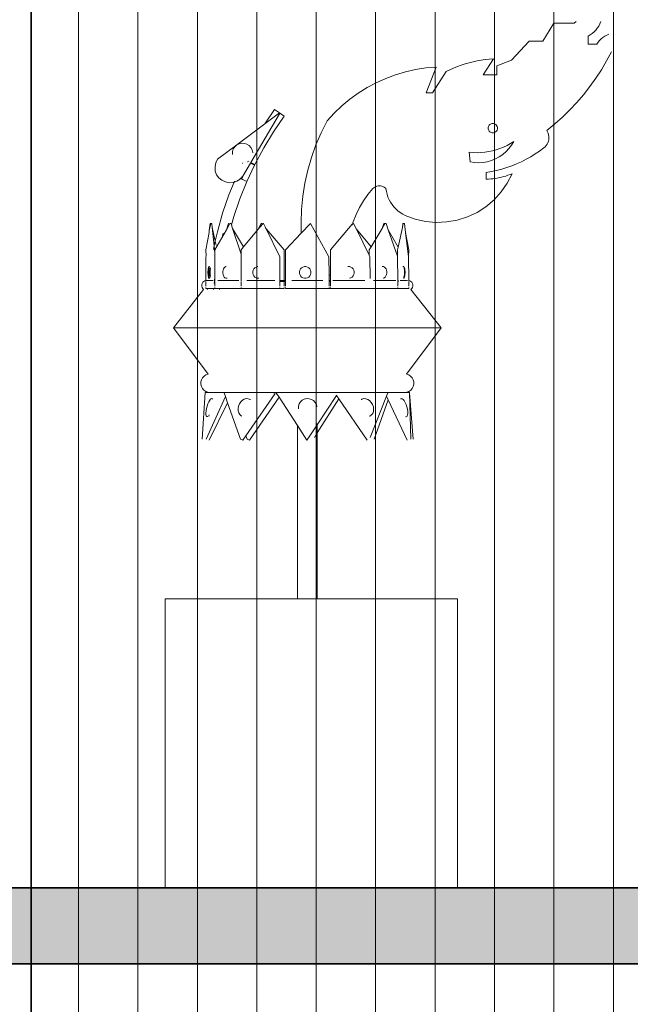
# Model space of a CAD drawing. Units: millimetres. Extents: x 446512 to 447461, y 70395 to 70610.
# Tile 24 of 39: x 446983 to 447016, y 70477 to 70530. Entities that reach past the tile are written whole.
import ezdxf

# ---------------------------------------------------------------- set-up
doc = ezdxf.new("R2010")
doc.units = ezdxf.units.MM
for name, color, linetype, lineweight in [('A-FURN', 7, 'Continuous', 35), ('A-FURN-DECO', 8, 'Continuous', 13), ('A-FURN-PATT', 38, 'Continuous', 13)]:
    doc.layers.add(name, color=color, linetype=linetype, lineweight=lineweight)

msp = doc.modelspace()

# ---------------------------------------------------------------- hatches: boundary and pattern name
at = {"layer": 'A-FURN-PATT'}
h = msp.add_hatch(dxfattribs=at)
h.set_pattern_fill('ANSI31', color=256, angle=45)
h.paths.add_polyline_path([(447044.0961, 70599.7147), (446983.5069, 70599.7147), (446983.5069, 70556.4508), (447030.1693, 70556.4508), (447030.1693, 70442.4508), (446983.5069, 70442.4508), (446983.5069, 70405.3145), (447044.0961, 70405.3145)])
h.paths.add_polyline_path([(447021.1693, 70547.4508), (446983.5069, 70547.4508), (446983.5069, 70451.4508), (447021.1693, 70451.4508)], flags=17)
h = msp.add_hatch(color=256, dxfattribs=at)
h.dxf.hatch_style = 1
h.paths.add_polyline_path([(447021.1693, 70483.6935), (446983.5069, 70483.6935), (446983.5069, 70479.6272), (447021.1693, 70479.6272)], flags=17)
h.paths.add_polyline_path([(447030.1693, 70483.6935), (447021.1693, 70483.6935), (447021.1693, 70479.6272), (447030.1693, 70479.6272)], flags=17)
h.paths.add_polyline_path([(447044.0961, 70599.7147), (446983.5069, 70599.7147), (446983.5069, 70556.4508), (447030.1693, 70556.4508), (447030.1693, 70442.4508), (446983.5069, 70442.4508), (446983.5069, 70405.3145), (447044.0961, 70405.3145)])
h = msp.add_hatch(color=256, dxfattribs=at)
h.dxf.hatch_style = 1
h.paths.add_polyline_path([(446983.5069, 70483.6935), (446973.1693, 70483.6935), (446973.1693, 70479.6272), (446983.5069, 70479.6272)])

# ---------------------------------------------------------------- linework, layer by layer
at = {"layer": 'A-FURN'}
for p, q in [((446983.5069, 70599.7147), (446983.5069, 70405.3145)), ((446990.6642, 70483.6935), (447006.2723, 70483.6935))]:
    msp.add_line(p, q, dxfattribs=at)
msp.add_lwpolyline([(446964.1693, 70483.6935), (447030.1693, 70483.6935), (447030.1693, 70479.6272), (446964.1693, 70479.6272)], close=True, dxfattribs=at)
at = {"layer": 'A-FURN-DECO'}
for p, q in [((447010.828, 70528.8929), (447011.4196, 70529.8484)), ((447011.4196, 70529.8484), (447012.5122, 70529.8484)), ((447012.5122, 70529.8484), (447012.6141, 70529.9403)), ((447013.7432, 70529.5803), (447013.6614, 70529.477)), ((447013.815, 70529.6908), (447013.7432, 70529.5803)), ((447013.8759, 70529.8076), (447013.815, 70529.6908)), ((447013.9256, 70529.9297), (447013.8759, 70529.8076)), ((447013.3629, 70529.2196), (447013.2487, 70529.1538)), ((447013.2487, 70529.1538), (447013.2487, 70528.7324)), ((447013.4704, 70529.2958), (447013.3629, 70529.2196)), ((447013.5702, 70529.3819), (447013.4704, 70529.2958)), ((447013.6614, 70529.477), (447013.5702, 70529.3819)), ((447013.8599, 70528.9241), (447013.9447, 70529.0087)), ((447013.9447, 70529.0087), (447014.0372, 70529.0847)), ((447014.0372, 70529.0847), (447014.1366, 70529.1514)), ((447014.1366, 70529.1514), (447014.242, 70529.2082)), ((447014.242, 70529.2082), (447014.3524, 70529.2545)), ((447009.1665, 70527.8803), (447010.0944, 70528.8929)), ((447010.0944, 70528.8929), (447010.828, 70528.8929)), ((447013.2487, 70528.7324), (447013.7169, 70528.7324)), ((447013.7169, 70528.7324), (447013.7838, 70528.8317)), ((447013.7838, 70528.8317), (447013.8599, 70528.9241)), ((447008.1897, 70527.9357), (447007.6509, 70527.0946)), ((447007.7535, 70527.9005), (447007.9713, 70527.922)), ((447007.9713, 70527.922), (447008.1897, 70527.9357)), ((447014.4944, 70528.3187), (447014.2376, 70527.8352)), ((447004.0349, 70527.3713), (447004.5847, 70527.4558)), ((447004.5847, 70527.4558), (447005.139, 70527.5027)), ((447005.139, 70527.5027), (447004.5947, 70526.1235)), ((447005.867, 70527.3633), (447006.0668, 70527.4527)), ((447006.0668, 70527.4527), (447006.2696, 70527.5349)), ((447006.2696, 70527.5349), (447006.4753, 70527.6097)), ((447006.4753, 70527.6097), (447006.6835, 70527.6771)), ((447006.6835, 70527.6771), (447006.8941, 70527.7371)), ((447006.8941, 70527.7371), (447007.1066, 70527.7894)), ((447007.1066, 70527.7894), (447007.3208, 70527.8342)), ((447007.3208, 70527.8342), (447007.5366, 70527.8712)), ((447007.5366, 70527.8712), (447007.7535, 70527.9005)), ((447008.3689, 70527.5628), (447009.1665, 70527.8803)), ((447008.3689, 70527.0946), (447008.3689, 70527.5628)), ((447014.2376, 70527.8352), (447013.9594, 70527.3635)), ((447001.9306, 70526.6685), (447002.4375, 70526.8975)), ((447002.4375, 70526.8975), (447002.9588, 70527.0915)), ((447002.9588, 70527.0915), (447003.4921, 70527.2497)), ((447003.4921, 70527.2497), (447004.0349, 70527.3713)), ((447004.9381, 70526.1235), (447005.6705, 70527.2669)), ((447005.6705, 70527.2669), (447005.867, 70527.3633)), ((447007.6509, 70527.0946), (447008.3689, 70527.0946)), ((447013.6605, 70526.9048), (447013.3415, 70526.4598)), ((447013.9594, 70527.3635), (447013.6605, 70526.9048)), ((447000.9691, 70526.1101), (447001.4403, 70526.4057)), ((447001.4403, 70526.4057), (447001.9306, 70526.6685)), ((447013.3415, 70526.4598), (447013.0029, 70526.0295)), ((447000.519, 70525.7833), (447000.9691, 70526.1101)), ((447004.5947, 70526.1235), (447004.9381, 70526.1235)), ((447013.0029, 70526.0295), (447012.6455, 70525.6147)), ((446999.6905, 70525.0418), (447000.0921, 70525.4266)), ((447000.0921, 70525.4266), (447000.519, 70525.7833)), ((447012.6455, 70525.6147), (447012.2699, 70525.2162)), ((446996.7604, 70525.015), (446995.2353, 70522.4145)), ((446996.5029, 70525.2318), (446995.9841, 70524.4744)), ((446996.7604, 70525.0554), (446995.9841, 70524.4744)), ((446996.4467, 70524.0451), (446997.018, 70524.879)), ((446996.7604, 70525.0554), (446996.5029, 70525.2318)), ((446996.7604, 70525.015), (446996.7604, 70525.0554)), ((446997.018, 70524.879), (446996.7604, 70525.0554)), ((446999.3159, 70524.6306), (446999.6905, 70525.0418)), ((447011.8769, 70524.8349), (447011.4674, 70524.4715)), ((447012.2699, 70525.2162), (447011.8769, 70524.8349)), ((446995.9841, 70524.4744), (446994.4826, 70523.344)), ((446999.3159, 70524.6306), (446998.9957, 70523.9976)), ((447007.9127, 70524.2101), (447007.913, 70524.2753)), ((447007.913, 70524.2753), (447007.9302, 70524.3381)), ((447007.9302, 70524.3381), (447007.9631, 70524.3944)), ((447007.9631, 70524.3944), (447008.0095, 70524.4403)), ((447008.0095, 70524.4403), (447008.0661, 70524.4726)), ((447008.0661, 70524.4726), (447008.1291, 70524.4891)), ((447008.1291, 70524.4891), (447008.1943, 70524.4888)), ((447008.1943, 70524.4888), (447008.2572, 70524.4716)), ((447008.2572, 70524.4716), (447008.3135, 70524.4387)), ((447008.3135, 70524.4387), (447008.3594, 70524.3924)), ((447008.3594, 70524.3924), (447008.3917, 70524.3358)), ((447008.3917, 70524.3358), (447008.4082, 70524.2727)), ((447008.4082, 70524.2727), (447008.4079, 70524.2075)), ((447011.4674, 70524.4715), (447011.042, 70524.1267)), ((446995.9258, 70523.1888), (446996.4467, 70524.0451)), ((446998.9957, 70523.9976), (446998.7153, 70523.3461)), ((447007.9292, 70524.147), (447007.9127, 70524.2101)), ((447007.9616, 70524.0904), (447007.9292, 70524.147)), ((447008.0074, 70524.044), (447007.9616, 70524.0904)), ((447008.0637, 70524.0112), (447008.0074, 70524.044)), ((447008.1266, 70523.994), (447008.0637, 70524.0112)), ((447008.1918, 70523.9936), (447008.1266, 70523.994)), ((447008.2548, 70524.0102), (447008.1918, 70523.9936)), ((447008.3115, 70524.0425), (447008.2548, 70524.0102)), ((447008.3578, 70524.0883), (447008.3115, 70524.0425)), ((447008.3907, 70524.1446), (447008.3578, 70524.0883)), ((447008.4079, 70524.2075), (447008.3907, 70524.1446)), ((447011.042, 70524.1267), (447011.0855, 70524.0511)), ((447011.0855, 70524.0511), (447011.1192, 70523.9707)), ((447011.1192, 70523.9707), (447011.1426, 70523.8866)), ((447011.1426, 70523.8866), (447011.1554, 70523.8004)), ((447011.1573, 70523.7131), (447011.1484, 70523.6264)), ((447011.1554, 70523.8004), (447011.1573, 70523.7131)), ((446994.4826, 70523.344), (446993.4537, 70522.5809)), ((446994.2989, 70523.1363), (446994.3766, 70523.2518)), ((446994.3766, 70523.2518), (446994.4826, 70523.344)), ((446994.4826, 70523.344), (446994.6097, 70523.4065)), ((446994.6097, 70523.4065), (446994.7492, 70523.4351)), ((446994.7492, 70523.4351), (446994.8916, 70523.4278)), ((446994.8916, 70523.4278), (446995.0273, 70523.3852)), ((446995.0273, 70523.3852), (446995.1468, 70523.3101)), ((446995.1468, 70523.3101), (446995.2422, 70523.2077)), ((446995.2422, 70523.2077), (446995.3069, 70523.085)), ((446995.9258, 70523.1888), (446995.4519, 70522.3056)), ((446998.7153, 70523.3461), (446998.4757, 70522.6785)), ((447008.7364, 70523.2332), (447008.5432, 70523.1548)), ((447008.9247, 70523.3227), (447008.7364, 70523.2332)), ((447009.1074, 70523.4232), (447008.9247, 70523.3227)), ((447009.1636, 70523.3387), (447009.0236, 70523.1569)), ((447009.2838, 70523.5343), (447009.1074, 70523.4232)), ((447009.2838, 70523.5343), (447009.1636, 70523.3387)), ((447010.8853, 70523.1876), (447010.6588, 70523.0208)), ((447010.951, 70523.245), (447010.8853, 70523.1876)), ((447011.009, 70523.3102), (447010.951, 70523.245)), ((447011.0584, 70523.3821), (447011.009, 70523.3102)), ((447011.0985, 70523.4595), (447011.0584, 70523.3821)), ((447011.1287, 70523.5414), (447011.0985, 70523.4595)), ((447011.1484, 70523.6264), (447011.1287, 70523.5414)), ((446994.2473, 70522.8678), (446994.2548, 70523.0053)), ((446994.2484, 70522.8629), (446994.2473, 70522.8678)), ((446994.2473, 70522.8435), (446994.2484, 70522.8629)), ((446994.2548, 70523.0053), (446994.2989, 70523.1363)), ((446995.3069, 70523.085), (446995.3365, 70522.9502)), ((446995.3355, 70522.9308), (446995.3365, 70522.9502)), ((446995.3355, 70522.9308), (446995.3365, 70522.926)), ((446998.4757, 70522.6785), (446998.2778, 70521.9974)), ((447007.1102, 70522.9384), (447006.9025, 70522.9561)), ((447006.9025, 70522.9561), (447006.9537, 70522.4376)), ((447007.3186, 70522.9328), (447007.1102, 70522.9384)), ((447007.527, 70522.9395), (447007.3186, 70522.9328)), ((447007.7346, 70522.9585), (447007.527, 70522.9395)), ((447007.9408, 70522.9896), (447007.7346, 70522.9585)), ((447008.1447, 70523.0329), (447007.9408, 70522.9896)), ((447008.3458, 70523.088), (447008.1447, 70523.0329)), ((447008.5004, 70522.7132), (447008.2982, 70522.6046)), ((447008.5432, 70523.1548), (447008.3458, 70523.088)), ((447008.6901, 70522.8424), (447008.5004, 70522.7132)), ((447008.8651, 70522.9908), (447008.6901, 70522.8424)), ((447009.0236, 70523.1569), (447008.8651, 70522.9908)), ((447010.1858, 70522.7165), (447009.9402, 70522.5794)), ((447010.4255, 70522.8637), (447010.1858, 70522.7165)), ((447010.6588, 70523.0208), (447010.4255, 70522.8637)), ((446993.3619, 70522.3972), (446993.3224, 70522.1968)), ((446993.3224, 70522.1564), (446993.3224, 70522.1968)), ((446993.3224, 70522.1564), (446993.338, 70521.953)), ((446993.4537, 70522.5809), (446993.3619, 70522.3972)), ((446994.7995, 70522.3847), (446994.7884, 70522.3611)), ((446995.2135, 70522.3774), (446994.8064, 70521.6831)), ((446995.0294, 70521.4043), (446995.4365, 70522.2728)), ((446995.0554, 70522.4515), (446995.0806, 70522.4397)), ((446995.1245, 70522.4701), (446995.1069, 70522.479)), ((446995.2353, 70522.4145), (446995.2135, 70522.3774)), ((446995.4365, 70522.2728), (446995.2135, 70522.3774)), ((446995.2353, 70522.4145), (446995.4519, 70522.3056)), ((447007.1809, 70522.4055), (447006.9537, 70522.4376)), ((447007.4103, 70522.3976), (447007.1809, 70522.4055)), ((447007.6393, 70522.4139), (447007.4103, 70522.3976)), ((447007.8652, 70522.4541), (447007.6393, 70522.4139)), ((447008.0857, 70522.518), (447007.8652, 70522.4541)), ((447008.2982, 70522.6046), (447008.0857, 70522.518)), ((447008.9067, 70522.1377), (447008.6379, 70522.0548)), ((447009.1718, 70522.2317), (447008.9067, 70522.1377)), ((447009.4327, 70522.3369), (447009.1718, 70522.2317)), ((447009.689, 70522.4528), (447009.4327, 70522.3369)), ((447009.9402, 70522.5794), (447009.689, 70522.4528)), ((446993.338, 70521.953), (446993.4076, 70521.7604)), ((446993.4076, 70521.7604), (446993.5263, 70521.5917)), ((446994.6967, 70521.5603), (446994.8064, 70521.6831)), ((446994.851, 70521.7593), (446994.7467, 70521.5369)), ((446998.2778, 70521.9974), (446998.1223, 70521.3053)), ((447008.0911, 70521.9232), (447007.814, 70521.8748)), ((447007.814, 70521.8748), (447007.814, 70521.5158)), ((447008.3659, 70521.9833), (447008.0911, 70521.9232)), ((447008.6379, 70522.0548), (447008.3659, 70521.9833)), ((447008.514, 70521.6004), (447008.6288, 70521.6265)), ((447008.6288, 70521.6265), (447008.7427, 70521.656)), ((447008.7427, 70521.656), (447008.8557, 70521.6889)), ((447008.8557, 70521.6889), (447008.9677, 70521.725)), ((447009.1882, 70521.8072), (447008.9299, 70521.3024)), ((447008.9677, 70521.725), (447009.0785, 70521.7645)), ((447009.0785, 70521.7645), (447009.1882, 70521.8072)), ((446993.5263, 70521.5917), (446993.6862, 70521.4585)), ((446993.6862, 70521.4585), (446993.8764, 70521.3698)), ((446993.8764, 70521.3698), (446994.0839, 70521.3317)), ((446994.3382, 70521.3615), (446994.0656, 70520.6874)), ((446994.0839, 70521.3317), (446994.2945, 70521.3467)), ((446994.2945, 70521.3467), (446994.3382, 70521.3615)), ((446994.3382, 70521.3615), (446994.4939, 70521.4139)), ((446994.3571, 70521.4083), (446994.3382, 70521.3615)), ((446994.4939, 70521.4139), (446994.6685, 70521.5287)), ((446994.6507, 70520.469), (446995.0265, 70521.3981)), ((446994.655, 70521.5602), (446994.685, 70521.5471)), ((446994.6685, 70521.5287), (446994.685, 70521.5471)), ((446994.6967, 70521.5603), (446994.6736, 70521.5711)), ((446994.685, 70521.5471), (446994.6967, 70521.5603)), ((446994.685, 70521.5471), (446995.0265, 70521.3981)), ((446994.6967, 70521.5603), (446995.0294, 70521.4043)), ((446994.7467, 70521.5369), (446994.7403, 70521.523)), ((446998.1223, 70521.3053), (446998.0099, 70520.605)), ((447001.8507, 70521.0987), (447001.7973, 70521.06)), ((447001.9089, 70521.1296), (447001.8507, 70521.0987)), ((447001.9708, 70521.1521), (447001.9089, 70521.1296)), ((447002.0353, 70521.1657), (447001.9708, 70521.1521)), ((447002.101, 70521.1703), (447002.0353, 70521.1657)), ((447002.1668, 70521.1657), (447002.101, 70521.1703)), ((447002.2313, 70521.1521), (447002.1668, 70521.1657)), ((447002.2932, 70521.1296), (447002.2313, 70521.1521)), ((447002.3514, 70521.0987), (447002.2932, 70521.1296)), ((447002.4048, 70521.06), (447002.3514, 70521.0987)), ((447007.814, 70521.5158), (447007.9315, 70521.5213)), ((447007.9315, 70521.5213), (447008.0489, 70521.5302)), ((447008.0489, 70521.5302), (447008.1659, 70521.5426)), ((447008.1659, 70521.5426), (447008.2825, 70521.5584)), ((447008.2825, 70521.5584), (447008.3986, 70521.5777)), ((447008.3986, 70521.5777), (447008.514, 70521.6004)), ((447008.9299, 70521.3024), (447008.6075, 70520.836)), ((446994.0656, 70520.6874), (446993.7296, 70519.7073)), ((446998.0099, 70520.605), (446997.941, 70519.899)), ((447001.4853, 70520.6969), (447001.2466, 70520.3596)), ((447001.7499, 70521.0143), (447001.4853, 70520.6969)), ((447001.7973, 70521.06), (447001.7499, 70521.0143)), ((447002.4522, 70521.0143), (447002.4048, 70521.06)), ((447002.4749, 70520.8621), (447002.4522, 70521.0143)), ((447002.5107, 70520.7125), (447002.4749, 70520.8621)), ((447002.5595, 70520.5666), (447002.5107, 70520.7125)), ((447002.6207, 70520.4254), (447002.5595, 70520.5666)), ((447008.6075, 70520.836), (447008.2264, 70520.4162)), ((446994.3256, 70519.5208), (446994.6507, 70520.469)), ((447001.2466, 70520.3596), (447001.0353, 70520.0045)), ((447002.694, 70520.2902), (447002.6207, 70520.4254)), ((447002.7787, 70520.1618), (447002.694, 70520.2902)), ((447002.8743, 70520.0413), (447002.7787, 70520.1618)), ((447002.9801, 70519.9295), (447002.8743, 70520.0413)), ((447007.7934, 70520.0502), (447007.3159, 70519.7444)), ((447008.2264, 70520.4162), (447007.7934, 70520.0502)), ((446993.7296, 70519.7073), (446993.447, 70518.7106)), ((446994.1992, 70519.0747), (446994.3256, 70519.5208)), ((446997.941, 70519.899), (446997.9158, 70519.1902)), ((447000.8526, 70519.6339), (447000.6997, 70519.2501)), ((447001.0353, 70520.0045), (447000.8526, 70519.6339)), ((447003.0951, 70519.8274), (447002.9801, 70519.9295)), ((447003.2186, 70519.7357), (447003.0951, 70519.8274)), ((447003.3497, 70519.6551), (447003.2186, 70519.7357)), ((447003.4872, 70519.5862), (447003.3497, 70519.6551)), ((447004.0189, 70519.3891), (447003.4872, 70519.5862)), ((447006.8023, 70519.5041), (447006.2615, 70519.3336)), ((447007.3159, 70519.7444), (447006.8023, 70519.5041)), ((446993.0154, 70518.7719), (446993.0649, 70519.161)), ((446993.0901, 70519.161), (446993.0154, 70518.7719)), ((446993.0901, 70519.161), (446993.0649, 70519.161)), ((446993.0901, 70519.161), (446993.1514, 70519.161)), ((446993.1746, 70518.9378), (446993.1514, 70519.161)), ((446993.93, 70518.8245), (446994.0469, 70519.161)), ((446994.1208, 70519.161), (446993.93, 70518.8245)), ((446994.0614, 70519.161), (446994.0469, 70519.161)), ((446994.1708, 70519.161), (446994.1208, 70519.161)), ((446994.1992, 70519.0747), (446994.1708, 70519.161)), ((446994.2625, 70518.8821), (446994.1992, 70519.0747)), ((446995.6281, 70518.8465), (446995.7833, 70519.161)), ((446995.8507, 70519.1138), (446995.6281, 70518.8465)), ((446995.8106, 70519.161), (446995.7833, 70519.161)), ((446995.8106, 70519.161), (446995.8507, 70519.1138)), ((446995.89, 70519.161), (446995.8507, 70519.1138)), ((446995.9197, 70519.161), (446995.89, 70519.161)), ((446996.0624, 70518.8653), (446995.9197, 70519.161)), ((446997.9158, 70519.1902), (446997.9304, 70518.636)), ((446998.4275, 70519.161), (446997.9304, 70518.636)), ((446999.4032, 70517.382), (446998.4275, 70519.161)), ((447000.6564, 70519.1101), (446999.4869, 70517.7442)), ((447000.6564, 70519.1101), (447000.6445, 70519.0715)), ((447000.6601, 70519.1218), (447000.6564, 70519.1101)), ((447000.6564, 70519.1101), (447000.6668, 70519.0976)), ((447000.6997, 70519.2501), (447000.6601, 70519.1218)), ((447000.6935, 70519.161), (447000.6601, 70519.1218)), ((447000.6935, 70519.161), (447000.7207, 70519.161)), ((447000.8759, 70518.8465), (447000.7207, 70519.161)), ((447002.2416, 70518.8821), (447002.3332, 70519.161)), ((447002.3957, 70519.139), (447002.2416, 70518.8821)), ((447002.3332, 70519.161), (447002.3832, 70519.161)), ((447002.3832, 70519.161), (447002.3957, 70519.139)), ((447002.4088, 70519.161), (447002.3957, 70519.139)), ((447002.4088, 70519.161), (447002.4572, 70519.161)), ((447002.5741, 70518.8245), (447002.4572, 70519.161)), ((447003.3295, 70518.9378), (447003.3526, 70519.161)), ((447003.3784, 70519.161), (447003.3295, 70518.9378)), ((447003.3526, 70519.161), (447003.3784, 70519.161)), ((447003.3784, 70519.161), (447003.4392, 70519.161)), ((447003.4392, 70519.161), (447003.501, 70518.6746)), ((447004.5718, 70519.2638), (447004.0189, 70519.3891)), ((447005.1365, 70519.2124), (447004.5718, 70519.2638)), ((447005.703, 70519.2358), (447005.1365, 70519.2124)), ((447006.2615, 70519.3336), (447005.703, 70519.2358)), ((446993.003, 70518.6746), (446992.8365, 70517.7442)), ((446993.003, 70518.6746), (446993.0154, 70518.7719)), ((446993.1746, 70518.9378), (446993.3341, 70518.2106)), ((446993.2765, 70517.9553), (446993.1746, 70518.9378)), ((446993.93, 70518.8245), (446993.3173, 70517.7442)), ((446993.447, 70518.7106), (446993.3341, 70518.2106)), ((446993.7497, 70518.6335), (446993.702, 70518.4225)), ((446994.2625, 70518.8821), (446994.8465, 70517.908)), ((446994.7101, 70517.5195), (446994.2625, 70518.8821)), ((446995.6281, 70518.8465), (446994.8465, 70517.908)), ((446995.9939, 70518.9457), (446996.0624, 70518.8653)), ((446996.0624, 70518.8653), (446997.0171, 70517.7442)), ((446996.7781, 70517.382), (446996.0624, 70518.8653)), ((446997.9304, 70518.636), (446997.0861, 70517.7442)), ((447000.8759, 70518.8465), (447001.6575, 70517.908)), ((447000.8759, 70518.8465), (447001.5593, 70517.4615)), ((447002.2416, 70518.8821), (447001.6575, 70517.908)), ((447002.5741, 70518.8245), (447003.1008, 70517.8957)), ((447002.5741, 70518.8245), (447003.0676, 70517.4039)), ((447003.3295, 70518.9378), (447003.1008, 70517.8957)), ((447003.501, 70518.6746), (447003.6675, 70517.7442)), ((447003.6653, 70517.382), (447003.501, 70518.6746)), ((446993.2765, 70517.9553), (446993.2345, 70517.7693)), ((446993.3341, 70518.2106), (446993.2765, 70517.9553)), ((446993.3173, 70517.5613), (446993.2765, 70517.9553)), ((446993.3341, 70518.2106), (446993.3803, 70518.0001)), ((446992.8365, 70517.7442), (446992.8416, 70517.4042)), ((446992.8387, 70517.382), (446992.8416, 70517.4042)), ((446993.3173, 70517.7442), (446993.3173, 70517.5613)), ((446993.3173, 70517.5613), (446993.3173, 70516.1152)), ((446994.8465, 70517.908), (446994.7101, 70517.7442)), ((446994.7101, 70517.7442), (446994.7101, 70517.5195)), ((446994.7101, 70517.5195), (446994.7101, 70516.0977)), ((446997.0171, 70517.7442), (446997.0171, 70516.1152)), ((446997.0861, 70517.7442), (446997.0861, 70516.1152)), ((446999.4869, 70517.7442), (446999.4869, 70516.3904)), ((447001.6575, 70517.908), (447001.5593, 70517.7442)), ((447001.5593, 70517.7442), (447001.5593, 70517.4615)), ((447001.5985, 70517.382), (447001.5593, 70517.4615)), ((447003.1008, 70517.8957), (447003.0676, 70517.7442)), ((447003.0676, 70517.7442), (447003.0676, 70517.4039)), ((447003.0752, 70517.382), (447003.0676, 70517.4039)), ((447003.6675, 70517.7442), (447003.6653, 70517.382)), ((446992.8387, 70517.382), (446992.8362, 70516.1111)), ((446996.7781, 70517.382), (446996.7877, 70516.1152)), ((446999.4032, 70517.382), (446999.4118, 70516.3898)), ((447001.5985, 70517.382), (447001.6076, 70516.2109)), ((447003.0752, 70517.382), (447003.0821, 70516.1152)), ((447003.6653, 70517.382), (447003.6678, 70516.1111)), ((446992.9462, 70516.5843), (446992.9502, 70516.6629)), ((446992.9462, 70516.5028), (446992.9462, 70516.5843)), ((446992.9501, 70516.424), (446992.9462, 70516.5028)), ((446992.9578, 70516.3533), (446992.9501, 70516.424)), ((446992.9502, 70516.6629), (446992.958, 70516.7334)), ((446992.9687, 70516.2956), (446992.9578, 70516.3533)), ((446992.958, 70516.7334), (446992.9689, 70516.7909)), ((446992.9689, 70516.7909), (446992.9823, 70516.8314)), ((446992.9768, 70516.5028), (446992.9769, 70516.5843)), ((446992.9808, 70516.424), (446992.9768, 70516.5028)), ((446992.9769, 70516.5843), (446992.9809, 70516.6629)), ((446992.9884, 70516.3533), (446992.9808, 70516.424)), ((446992.9809, 70516.6629), (446992.9886, 70516.7334)), ((446992.9823, 70516.8314), (446992.9972, 70516.8523)), ((446992.9993, 70516.2956), (446992.9884, 70516.3533)), ((446992.9886, 70516.7334), (446992.9996, 70516.7909)), ((446993.0278, 70516.8523), (446992.9972, 70516.8523)), ((446993.0299, 70516.5011), (446992.9993, 70516.2956)), ((446992.9996, 70516.7909), (446993.0129, 70516.8314)), ((446993.0129, 70516.8314), (446993.0278, 70516.8523)), ((446993.0347, 70516.6614), (446993.0298, 70516.5826)), ((446993.0298, 70516.5826), (446993.0299, 70516.5011)), ((446993.0299, 70516.5011), (446993.0348, 70516.4225)), ((446993.0441, 70516.7321), (446993.0347, 70516.6614)), ((446993.0455, 70516.6785), (446993.0347, 70516.6614)), ((446993.0348, 70516.4225), (446993.0443, 70516.352)), ((446993.0574, 70516.7898), (446993.0441, 70516.7321)), ((446993.0441, 70516.7321), (446993.0455, 70516.6785)), ((446993.0443, 70516.352), (446993.0577, 70516.2945)), ((446993.0651, 70516.8092), (446993.0574, 70516.7898)), ((446993.0668, 70516.8041), (446993.0574, 70516.7898)), ((446993.0651, 70516.6614), (446993.0602, 70516.5826)), ((446993.0602, 70516.5826), (446993.0603, 70516.5011)), ((446993.0603, 70516.5011), (446993.0652, 70516.4225)), ((446993.0745, 70516.7321), (446993.0651, 70516.6614)), ((446993.0652, 70516.4225), (446993.0747, 70516.352)), ((446993.0788, 70516.7508), (446993.0745, 70516.7321)), ((446993.0747, 70516.352), (446993.0788, 70516.3345)), ((446993.7369, 70516.5028), (446993.7371, 70516.5843)), ((446993.7494, 70516.424), (446993.7369, 70516.5028)), ((446993.7371, 70516.5843), (446993.7498, 70516.6629)), ((446993.7737, 70516.3533), (446993.7494, 70516.424)), ((446993.7498, 70516.6629), (446993.7743, 70516.7334)), ((446993.8082, 70516.2956), (446993.7737, 70516.3533)), ((446993.7743, 70516.7334), (446993.8089, 70516.7909)), ((446993.8089, 70516.7909), (446993.8513, 70516.8314)), ((446993.8513, 70516.8314), (446993.8985, 70516.8523)), ((446993.9235, 70516.8523), (446993.8985, 70516.8523)), ((446995.3482, 70516.5028), (446995.3484, 70516.5843)), ((446995.3665, 70516.424), (446995.3482, 70516.5028)), ((446995.3484, 70516.5843), (446995.3671, 70516.6629)), ((446995.4022, 70516.3533), (446995.3665, 70516.424)), ((446995.3671, 70516.6629), (446995.4031, 70516.7334)), ((446995.4528, 70516.2956), (446995.4022, 70516.3533)), ((446995.4031, 70516.7334), (446995.4539, 70516.7909)), ((446995.4539, 70516.7909), (446995.5161, 70516.8314)), ((446995.5161, 70516.8314), (446995.5854, 70516.8523)), ((446995.6002, 70516.8523), (446995.5854, 70516.8523)), ((446997.8283, 70516.5028), (446997.8285, 70516.5843)), ((446997.8492, 70516.424), (446997.8283, 70516.5028)), ((446997.8285, 70516.5843), (446997.8498, 70516.6629)), ((446997.8898, 70516.3533), (446997.8492, 70516.424)), ((446997.8498, 70516.6629), (446997.8908, 70516.7334)), ((446997.9472, 70516.2956), (446997.8898, 70516.3533)), ((446997.8908, 70516.7334), (446997.9485, 70516.7909)), ((446997.9485, 70516.7909), (446998.0192, 70516.8314)), ((446998.0192, 70516.8314), (446998.098, 70516.8523)), ((446998.098, 70516.8523), (446998.1795, 70516.8521)), ((446998.1795, 70516.8521), (446998.2581, 70516.8308)), ((446998.2581, 70516.8308), (446998.3286, 70516.7898)), ((446998.3851, 70516.352), (446998.3273, 70516.2945)), ((446998.3286, 70516.7898), (446998.3861, 70516.7321)), ((446998.426, 70516.4225), (446998.3851, 70516.352)), ((446998.3861, 70516.7321), (446998.4266, 70516.6614)), ((446998.4473, 70516.5011), (446998.426, 70516.4225)), ((446998.4266, 70516.6614), (446998.4475, 70516.5826)), ((446998.4475, 70516.5826), (446998.4473, 70516.5011)), ((446999.4869, 70516.3904), (446999.4118, 70516.3898)), ((446999.4118, 70516.3898), (446999.4141, 70516.1152)), ((446999.5141, 70516.3907), (446999.4869, 70516.3904)), ((446999.4869, 70516.3904), (446999.4869, 70516.1152)), ((447000.2282, 70516.3968), (447000.2147, 70516.3967)), ((447000.4244, 70516.8523), (447000.438, 70516.8523)), ((447000.438, 70516.8523), (447000.5113, 70516.8521)), ((447000.5113, 70516.8521), (447000.5821, 70516.8308)), ((447000.5821, 70516.8308), (447000.6455, 70516.7898)), ((447000.6962, 70516.352), (447000.6443, 70516.2945)), ((447000.6455, 70516.7898), (447000.6972, 70516.7321)), ((447000.7331, 70516.4225), (447000.6962, 70516.352)), ((447000.6972, 70516.7321), (447000.7336, 70516.6614)), ((447000.7522, 70516.5011), (447000.7331, 70516.4225)), ((447000.7336, 70516.6614), (447000.7524, 70516.5826)), ((447000.7524, 70516.5826), (447000.7522, 70516.5011)), ((447002.2485, 70516.8523), (447002.2726, 70516.8523)), ((447002.2726, 70516.8523), (447002.3243, 70516.8521)), ((447002.3243, 70516.8521), (447002.3741, 70516.8308)), ((447002.3741, 70516.8308), (447002.4187, 70516.7898)), ((447002.4545, 70516.352), (447002.4179, 70516.2945)), ((447002.4187, 70516.7898), (447002.4551, 70516.7321)), ((447002.4804, 70516.4225), (447002.4545, 70516.352)), ((447002.4551, 70516.7321), (447002.4808, 70516.6614)), ((447002.4939, 70516.5011), (447002.4804, 70516.4225)), ((447002.4808, 70516.6614), (447002.494, 70516.5826)), ((447002.494, 70516.5826), (447002.4939, 70516.5011)), ((447003.3628, 70516.8523), (447003.3817, 70516.8521)), ((447003.3817, 70516.8521), (447003.3932, 70516.8523)), ((447003.3817, 70516.8521), (447003.3999, 70516.8308)), ((447003.3932, 70516.8523), (447003.4121, 70516.8521)), ((447003.3999, 70516.8308), (447003.4163, 70516.7898)), ((447003.4121, 70516.8521), (447003.4303, 70516.8308)), ((447003.4293, 70516.352), (447003.4159, 70516.2945)), ((447003.4163, 70516.7898), (447003.4296, 70516.7321)), ((447003.4388, 70516.4225), (447003.4293, 70516.352)), ((447003.4296, 70516.7321), (447003.439, 70516.6614)), ((447003.4303, 70516.8308), (447003.4466, 70516.7898)), ((447003.4438, 70516.5011), (447003.4388, 70516.4225)), ((447003.439, 70516.6614), (447003.4438, 70516.5826)), ((447003.4438, 70516.5826), (447003.4438, 70516.5011)), ((447003.4597, 70516.352), (447003.4463, 70516.2945)), ((447003.4466, 70516.7898), (447003.4599, 70516.7321)), ((447003.4692, 70516.4225), (447003.4597, 70516.352)), ((447003.4599, 70516.7321), (447003.4693, 70516.6614)), ((447003.4741, 70516.5011), (447003.4692, 70516.4225)), ((447003.4693, 70516.6614), (447003.4742, 70516.5826)), ((447003.4742, 70516.5826), (447003.4741, 70516.5011)), ((446992.6127, 70515.8121), (446992.6137, 70515.8834)), ((446992.6137, 70515.8834), (446992.6332, 70515.952)), ((446992.6332, 70515.952), (446992.6697, 70516.0133)), ((446992.6697, 70516.0133), (446992.7208, 70516.063)), ((446992.7208, 70516.063), (446992.7831, 70516.0977)), ((446992.7831, 70516.0977), (446992.8362, 70516.1111)), ((446992.8361, 70516.063), (446992.8356, 70515.8121)), ((446992.8362, 70516.1111), (446992.8522, 70516.1152)), ((446992.8362, 70516.1111), (446992.8362, 70516.0977)), ((446992.8522, 70516.1152), (446992.8643, 70516.115)), ((446992.8522, 70516.1152), (446992.8571, 70516.1152)), ((446993.2179, 70516.1152), (446992.8643, 70516.115)), ((446992.982, 70516.2546), (446992.9687, 70516.2956)), ((446992.9968, 70516.2333), (446992.982, 70516.2546)), ((446993.0123, 70516.2331), (446992.9968, 70516.2333)), ((446993.0126, 70516.2546), (446992.9993, 70516.2956)), ((446993.0275, 70516.2333), (446993.0123, 70516.2331)), ((446993.0275, 70516.2333), (446993.0126, 70516.2546)), ((446993.0429, 70516.2331), (446993.0275, 70516.2333)), ((446993.0577, 70516.2945), (446993.0651, 70516.2762)), ((446993.3173, 70516.1152), (446993.2767, 70516.1152)), ((446993.3173, 70516.0582), (446993.2768, 70516.0582)), ((446993.2892, 70516.063), (446993.277, 70515.9561)), ((446993.3173, 70516.3088), (446993.2932, 70516.0977)), ((446993.3173, 70516.1152), (446993.3173, 70516.0977)), ((446993.3173, 70516.063), (446993.3173, 70516.0582)), ((446993.3173, 70516.0582), (446993.3173, 70515.8121)), ((446994.5923, 70516.1152), (446993.4652, 70516.1152)), ((446993.8504, 70516.2546), (446993.8082, 70516.2956)), ((446993.8975, 70516.2333), (446993.8504, 70516.2546)), ((446993.9463, 70516.2331), (446993.8975, 70516.2333)), ((446993.9713, 70516.2331), (446993.9463, 70516.2331)), ((446994.7101, 70516.063), (446994.7101, 70515.8121)), ((446995.0145, 70516.1152), (446996.5153, 70516.1152)), ((446995.5147, 70516.2546), (446995.4528, 70516.2956)), ((446995.5839, 70516.2333), (446995.5147, 70516.2546)), ((446995.6556, 70516.2331), (446995.5839, 70516.2333)), ((446995.6705, 70516.2331), (446995.6556, 70516.2331)), ((446996.7877, 70516.1152), (446996.758, 70516.1152)), ((446996.7881, 70516.0582), (446996.7584, 70516.0582)), ((446996.7877, 70516.1152), (446996.7878, 70516.0977)), ((446997.0171, 70516.1152), (446996.7877, 70516.1152)), ((446996.7881, 70516.063), (446996.7881, 70516.0582)), ((446996.7881, 70516.0582), (446996.79, 70515.8121)), ((446997.0171, 70516.0582), (446996.7881, 70516.0582)), ((446997.0171, 70516.1152), (446997.0861, 70516.1152)), ((446997.0171, 70516.1152), (446997.0171, 70516.0977)), ((446997.0171, 70516.063), (446997.0171, 70516.0582)), ((446997.0171, 70516.0582), (446997.0171, 70515.8121)), ((446997.0861, 70516.0582), (446997.0171, 70516.0582)), ((446997.0861, 70516.1152), (446997.0861, 70516.0977)), ((446997.0861, 70516.063), (446997.0861, 70516.0582)), ((446997.0861, 70516.0582), (446997.0861, 70515.8121)), ((446997.422, 70516.1152), (446999.082, 70516.1152)), ((446998.0177, 70516.2546), (446997.9472, 70516.2956)), ((446998.0963, 70516.2333), (446998.0177, 70516.2546)), ((446998.1778, 70516.2331), (446998.0963, 70516.2333)), ((446998.2566, 70516.254), (446998.1778, 70516.2331)), ((446998.3273, 70516.2945), (446998.2566, 70516.254)), ((446999.4141, 70516.1152), (446999.4143, 70516.0977)), ((446999.4869, 70516.1152), (446999.4141, 70516.1152)), ((446999.4146, 70516.063), (446999.4146, 70516.0582)), ((446999.4146, 70516.0582), (446999.4168, 70515.8121)), ((446999.4869, 70516.0582), (446999.4146, 70516.0582)), ((446999.5141, 70516.1152), (446999.4869, 70516.1152)), ((446999.4869, 70516.1152), (446999.4869, 70516.0977)), ((446999.4869, 70516.063), (446999.4869, 70516.0582)), ((446999.5141, 70516.0582), (446999.4869, 70516.0582)), ((446999.4869, 70516.0582), (446999.4869, 70515.8121)), ((446999.6124, 70516.1152), (447001.3285, 70516.1152)), ((447000.4962, 70516.2331), (447000.5098, 70516.2331)), ((447000.5807, 70516.254), (447000.5098, 70516.2331)), ((447000.6443, 70516.2945), (447000.5807, 70516.254)), ((447002.9791, 70516.1152), (447001.7834, 70516.1152)), ((447002.299, 70516.2331), (447002.3232, 70516.2331)), ((447002.3731, 70516.254), (447002.3232, 70516.2331)), ((447002.4179, 70516.2945), (447002.3731, 70516.254)), ((447003.1283, 70516.1152), (447003.0821, 70516.1152)), ((447003.0821, 70516.1152), (447003.0822, 70516.0977)), ((447003.0824, 70516.063), (447003.0824, 70516.0582)), ((447003.1283, 70516.0582), (447003.0824, 70516.0582)), ((447003.0824, 70516.0582), (447003.0838, 70515.8121)), ((447003.2085, 70516.1152), (447003.6039, 70516.1152)), ((447003.3996, 70516.254), (447003.3813, 70516.2331)), ((447003.3813, 70516.2331), (447003.4117, 70516.2331)), ((447003.4159, 70516.2945), (447003.3996, 70516.254)), ((447003.4299, 70516.254), (447003.4117, 70516.2331)), ((447003.4463, 70516.2945), (447003.4299, 70516.254)), ((447003.6678, 70516.1111), (447003.6675, 70516.0977)), ((447003.6675, 70516.063), (447003.6675, 70515.8121)), ((447003.6678, 70516.1111), (447003.7209, 70516.0977)), ((447003.7209, 70516.0977), (447003.7832, 70516.063)), ((447003.7832, 70516.063), (447003.8343, 70516.0133)), ((447003.8343, 70516.0133), (447003.8709, 70515.952)), ((447003.8709, 70515.952), (447003.8903, 70515.8834)), ((447003.8903, 70515.8834), (447003.8913, 70515.8121)), ((446991.0984, 70513.5846), (446992.7146, 70515.6296)), ((446992.6302, 70515.743), (446992.6127, 70515.8121)), ((446992.6649, 70515.6808), (446992.6302, 70515.743)), ((446992.7146, 70515.6296), (446992.6649, 70515.6808)), ((446992.8355, 70515.743), (446992.8353, 70515.6808)), ((446992.8416, 70515.6808), (446992.8353, 70515.6808)), ((446992.9312, 70515.6808), (446992.8353, 70515.6808)), ((446992.9276, 70515.6492), (446992.9264, 70515.6296)), ((446992.9312, 70515.6808), (446992.9276, 70515.6492)), ((446993.3173, 70515.6808), (446992.9312, 70515.6808)), ((446993.2454, 70515.6808), (446993.2396, 70515.6296)), ((446993.3173, 70515.743), (446993.3173, 70515.6808)), ((446993.3173, 70515.6808), (446993.5596, 70515.6808)), ((446993.5538, 70515.6296), (446993.5596, 70515.6808)), ((446993.5596, 70515.6808), (446994.7141, 70515.6808)), ((446994.7101, 70515.743), (446994.7141, 70515.6808)), ((446994.7141, 70515.6808), (446996.791, 70515.6808)), ((446996.7905, 70515.743), (446996.791, 70515.6808)), ((446997.0171, 70515.6808), (446996.791, 70515.6808)), ((446997.0171, 70515.743), (446997.0171, 70515.6808)), ((446997.0861, 70515.743), (446997.0861, 70515.6808)), ((446997.0861, 70515.6808), (446999.4179, 70515.6808)), ((446999.4174, 70515.743), (446999.4179, 70515.6808)), ((446999.4869, 70515.6808), (446999.4179, 70515.6808)), ((446999.4869, 70515.743), (446999.4869, 70515.6808)), ((447003.0845, 70515.6808), (446999.4869, 70515.6808)), ((447003.0841, 70515.743), (447003.0845, 70515.6808)), ((447003.6675, 70515.6808), (447003.0845, 70515.6808)), ((447003.6675, 70515.743), (447003.6675, 70515.6808)), ((447003.8391, 70515.6808), (447003.7894, 70515.6296)), ((447003.7894, 70515.6296), (447005.4056, 70513.5846)), ((447003.8739, 70515.743), (447003.8391, 70515.6808)), ((447003.8913, 70515.8121), (447003.8739, 70515.743)), ((446992.9486, 70511.1093), (446991.0984, 70513.5846)), ((447005.4056, 70513.5846), (446991.0984, 70513.5846)), ((447005.4056, 70513.5846), (447003.5554, 70511.1093)), ((446992.8356, 70511.0697), (446992.9486, 70511.1093)), ((447003.5554, 70511.1093), (447003.6684, 70511.0697)), ((446992.5642, 70510.5759), (446992.566, 70510.6956)), ((446992.5914, 70510.4593), (446992.5642, 70510.5759)), ((446992.566, 70510.6956), (446992.5966, 70510.8113)), ((446992.5966, 70510.8113), (446992.6542, 70510.9162)), ((446992.6542, 70510.9162), (446992.7355, 70511.0041)), ((446992.7355, 70511.0041), (446992.8356, 70511.0697)), ((447003.6684, 70511.0697), (447003.7685, 70511.0041)), ((447003.7685, 70511.0041), (447003.8498, 70510.9162)), ((447003.8498, 70510.9162), (447003.9075, 70510.8113)), ((447003.9075, 70510.8113), (447003.9381, 70510.6956)), ((447003.9398, 70510.5759), (447003.9126, 70510.4593)), ((447003.9381, 70510.6956), (447003.9398, 70510.5759)), ((446992.646, 70510.3528), (446992.5914, 70510.4593)), ((446992.6291, 70507.6484), (446992.8015, 70510.1366)), ((446992.7246, 70510.2625), (446992.646, 70510.3528)), ((446992.8228, 70510.194), (446992.7246, 70510.2625)), ((446993.0534, 70510.1366), (446992.8015, 70510.1366)), ((446992.9345, 70510.1511), (446992.8228, 70510.194)), ((446993.0534, 70510.1366), (446992.9345, 70510.1511)), ((446993.0534, 70510.1366), (446993.7498, 70510.1366)), ((446993.7498, 70510.1366), (446993.7975, 70510.1366)), ((446993.8035, 70510.1199), (446993.7498, 70510.1366)), ((446993.8035, 70510.1199), (446993.7975, 70510.1366)), ((446993.7975, 70510.1366), (446996.4058, 70510.1366)), ((446993.8745, 70509.9206), (446993.8035, 70510.1199)), ((446994.9736, 70507.8254), (446996.5338, 70510.08)), ((446996.4058, 70510.1366), (446996.6125, 70510.1366)), ((446996.5338, 70510.08), (446996.4058, 70510.1366)), ((446996.6125, 70510.08), (446996.6125, 70510.1366)), ((446999.5975, 70510.1366), (446996.6125, 70510.1366)), ((446996.7442, 70509.8781), (446996.6125, 70510.08)), ((446999.8581, 70510.134), (446999.5975, 70510.1366)), ((446999.8581, 70510.134), (446999.8636, 70510.1366)), ((446999.8636, 70510.1366), (446999.8762, 70510.1366)), ((447002.5608, 70510.1366), (446999.8762, 70510.1366)), ((447002.4823, 70509.9414), (447002.5522, 70510.1183)), ((447002.5522, 70510.1183), (447002.6166, 70510.1366)), ((447002.5522, 70510.1183), (447002.5608, 70510.1366)), ((447002.5608, 70510.1366), (447002.6166, 70510.1366)), ((447002.6166, 70510.1366), (447003.4507, 70510.1366)), ((447003.5695, 70510.1511), (447003.4507, 70510.1366)), ((447003.69, 70510.134), (447003.4507, 70510.1366)), ((447003.6813, 70510.194), (447003.5695, 70510.1511)), ((447003.7794, 70510.2625), (447003.6813, 70510.194)), ((447003.6994, 70510.1366), (447003.69, 70510.134)), ((447003.7012, 70510.1158), (447003.6994, 70510.1366)), ((447003.9113, 70507.6484), (447003.7012, 70510.1158)), ((447003.7821, 70507.6484), (447003.7012, 70510.1158)), ((447003.8581, 70510.3528), (447003.7794, 70510.2625)), ((447003.9126, 70510.4593), (447003.8581, 70510.3528)), ((446992.8525, 70507.6391), (446993.8745, 70509.9206)), ((446992.9006, 70509.4003), (446992.9423, 70509.521)), ((446992.9423, 70509.521), (446992.9895, 70509.6283)), ((446992.9895, 70509.6283), (446993.0389, 70509.7148)), ((446993.0158, 70507.5919), (446993.9957, 70509.5805)), ((446993.0389, 70509.7148), (446993.0873, 70509.7747)), ((446993.0873, 70509.7747), (446993.1312, 70509.8039)), ((446993.1312, 70509.8039), (446993.1677, 70509.8003)), ((446993.1745, 70509.7917), (446993.1677, 70509.8003)), ((446993.1745, 70509.7917), (446993.2111, 70509.7882)), ((446993.9957, 70509.5805), (446993.8745, 70509.9206)), ((446994.6841, 70507.6484), (446993.9957, 70509.5805)), ((446994.5746, 70509.4003), (446994.6239, 70509.521)), ((446994.6239, 70509.521), (446994.6957, 70509.6283)), ((446994.6957, 70509.6283), (446994.7851, 70509.7148)), ((446994.7851, 70509.7148), (446994.8861, 70509.7747)), ((446994.8861, 70509.7747), (446994.9917, 70509.8039)), ((446994.9917, 70509.8039), (446995.0948, 70509.8003)), ((446995.0948, 70509.8003), (446995.1917, 70509.7614)), ((446995.162, 70507.5919), (446996.7442, 70509.8781)), ((446995.1917, 70509.7614), (446995.2157, 70509.7522)), ((446997.7213, 70508.3795), (446996.7442, 70509.8781)), ((446997.7767, 70509.4003), (446997.8139, 70509.521)), ((446997.8139, 70509.521), (446997.8823, 70509.6283)), ((446997.8823, 70509.6283), (446997.977, 70509.7148)), ((446997.977, 70509.7148), (446998.0917, 70509.7747)), ((446998.0917, 70509.7747), (446998.2186, 70509.8039)), ((446998.2186, 70509.8039), (446998.3489, 70509.8003)), ((446998.3489, 70509.8003), (446998.4739, 70509.7643)), ((446998.4739, 70509.7643), (446998.5849, 70509.6983)), ((446998.5849, 70509.6983), (446998.6745, 70509.6068)), ((446998.6745, 70509.6068), (446998.7365, 70509.496)), ((446998.7827, 70508.4146), (446999.8187, 70509.9707)), ((446998.7827, 70507.979), (446999.9412, 70509.7929)), ((446999.8187, 70509.9707), (446999.7996, 70509.9985)), ((446999.9412, 70509.7929), (446999.8187, 70509.9707)), ((447001.4568, 70507.5919), (446999.9412, 70509.7929)), ((447001.1368, 70509.7626), (447001.1513, 70509.7668)), ((447001.1513, 70509.7668), (447001.1625, 70509.7747)), ((447001.1625, 70509.7747), (447001.2624, 70509.8039)), ((447001.2624, 70509.8039), (447001.3701, 70509.8003)), ((447001.3701, 70509.8003), (447001.4783, 70509.7643)), ((447001.4783, 70509.7643), (447001.5796, 70509.6983)), ((447001.5796, 70509.6983), (447001.6672, 70509.6068)), ((447001.6074, 70507.7255), (447002.4823, 70509.9414)), ((447001.6672, 70509.6068), (447001.7351, 70509.496)), ((447001.8281, 70507.6484), (447002.5735, 70509.7468)), ((447002.5735, 70509.7468), (447002.4823, 70509.9414)), ((447003.5829, 70507.5919), (447002.5735, 70509.7468)), ((447003.2347, 70509.7917), (447003.2774, 70509.8039)), ((447003.2347, 70509.7917), (447003.2605, 70509.7897)), ((447003.2774, 70509.8039), (447003.3213, 70509.8003)), ((447003.3213, 70509.8003), (447003.3717, 70509.7643)), ((447003.3717, 70509.7643), (447003.4251, 70509.6983)), ((447003.4251, 70509.6983), (447003.4779, 70509.6068)), ((447003.4779, 70509.6068), (447003.5264, 70509.496)), ((446992.8339, 70509.0411), (446992.8445, 70509.1519)), ((446992.8361, 70508.9496), (446992.8339, 70509.0411)), ((446992.8445, 70509.1519), (446992.8673, 70509.2745)), ((446992.8673, 70509.2745), (446992.9006, 70509.4003)), ((446994.5513, 70509.2745), (446994.5746, 70509.4003)), ((446994.5554, 70509.1519), (446994.5513, 70509.2745)), ((446994.5867, 70509.0411), (446994.5554, 70509.1519)), ((446994.6431, 70508.9496), (446994.5867, 70509.0411)), ((446997.773, 70509.2623), (446997.7733, 70509.2732)), ((446997.7733, 70509.2732), (446997.7767, 70509.4003)), ((446998.7365, 70509.496), (446998.7667, 70509.3735)), ((446998.7667, 70509.3614), (446998.7667, 70509.3735)), ((447001.7427, 70509.0196), (447001.678, 70508.9331)), ((447001.7351, 70509.496), (447001.7786, 70509.3735)), ((447001.7826, 70509.1269), (447001.7427, 70509.0196)), ((447001.7786, 70509.3735), (447001.7948, 70509.2476)), ((447001.7948, 70509.2476), (447001.7826, 70509.1269)), ((447003.5264, 70509.496), (447003.5673, 70509.3735)), ((447003.5673, 70509.3735), (447003.598, 70509.2476)), ((447003.598, 70509.2476), (447003.6162, 70509.1269)), ((447003.6207, 70509.0196), (447003.6113, 70508.9331)), ((447003.6162, 70509.1269), (447003.6207, 70509.0196)), ((446992.8511, 70508.8836), (446992.8361, 70508.9496)), ((446992.8778, 70508.8476), (446992.8511, 70508.8836)), ((446992.9146, 70508.8443), (446992.8778, 70508.8476)), ((446992.9211, 70508.8355), (446992.9146, 70508.8443)), ((446992.9845, 70508.9057), (446992.9997, 70508.8732)), ((446992.9997, 70508.8732), (446993.0071, 70508.8679)), ((446993.0105, 70508.9399), (446993.0135, 70508.921)), ((446994.7207, 70508.8836), (446994.6431, 70508.9496)), ((446994.7481, 70508.8715), (446994.7207, 70508.8836)), ((446998.7827, 70508.4146), (446998.7827, 70508.4712)), ((447001.5783, 70508.869), (447001.5671, 70508.8611)), ((447001.5783, 70508.869), (447001.5929, 70508.8732)), ((447001.678, 70508.9331), (447001.5929, 70508.8732)), ((447003.5281, 70508.8462), (447003.5113, 70508.832)), ((447003.5113, 70508.832), (447003.554, 70508.8441)), ((447003.5885, 70508.8732), (447003.554, 70508.8441)), ((447003.6113, 70508.9331), (447003.5885, 70508.8732)), ((446997.7213, 70499.1173), (446997.7213, 70508.3795)), ((446998.2349, 70507.5919), (446997.7213, 70508.3795)), ((446998.3839, 70507.8156), (446998.7827, 70508.4146)), ((446998.6273, 70507.7357), (446998.7827, 70507.979)), ((446998.7827, 70507.979), (446998.7827, 70508.4146)), ((446998.7827, 70499.1173), (446998.7827, 70507.979)), ((446994.812, 70507.5919), (446994.6841, 70507.6484)), ((446994.812, 70507.5919), (446994.9736, 70507.8254)), ((446995.0461, 70507.6484), (446994.9736, 70507.8254)), ((446995.162, 70507.5919), (446995.0461, 70507.6484)), ((446998.2349, 70507.5919), (446998.3839, 70507.8156)), ((446998.3839, 70507.8156), (446998.3649, 70507.8436)), ((446998.3894, 70507.8074), (446998.3839, 70507.8156)), ((446990.6642, 70483.6935), (446990.6642, 70499.1173)), ((446990.6642, 70499.1173), (446997.7213, 70499.1173)), ((446998.7827, 70499.1173), (446997.7213, 70499.1173)), ((446998.7827, 70499.1173), (447006.2723, 70499.1173)), ((447006.2723, 70483.6935), (447006.2723, 70499.1173))]:
    msp.add_line(p, q, dxfattribs=at)

doc.saveas('drawing.dxf')
